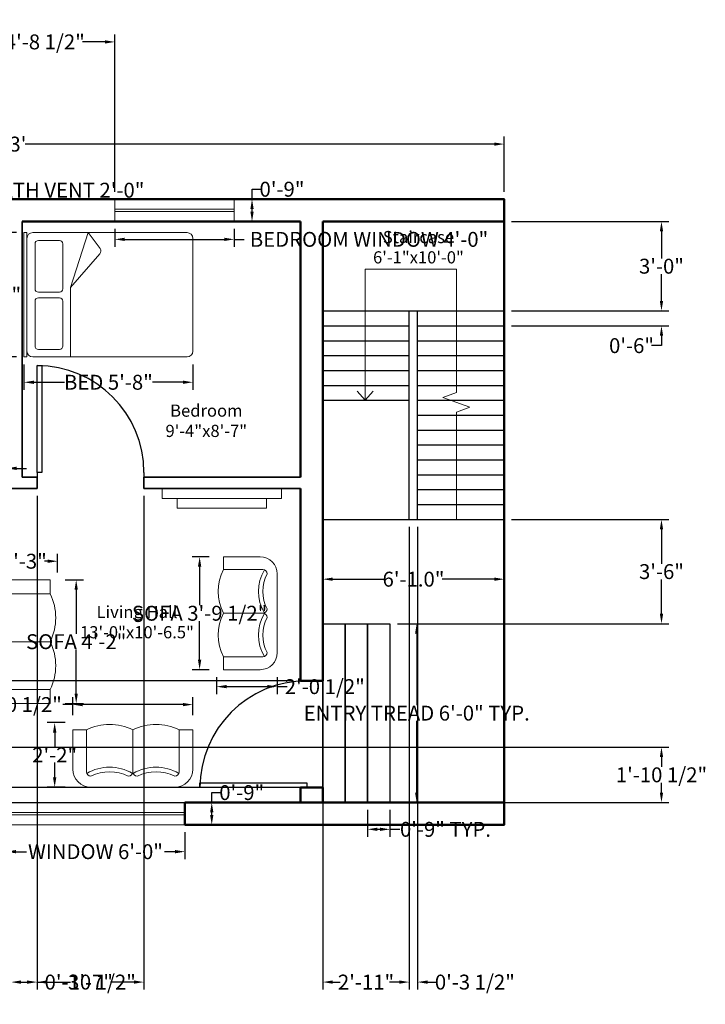
# Model space of a CAD drawing. Units: inches. Extents: x -59 to 502, y -260 to 136.
# Tile 8 of 8: x 226 to 502, y -260 to 136. Entities that reach past the tile are written whole.
import ezdxf

# ---------------------------------------------------------------- set-up
doc = ezdxf.new("R2010")
doc.units = ezdxf.units.IN
doc.header["$MEASUREMENT"] = 0
for name, color, linetype, lineweight in [('A-ANNO-DIMS', 2, 'Continuous', 18), ('A-ANNO-SYMB', 7, 'Continuous', 18), ('A-AREA-IDEN', 7, 'Continuous', 25), ('A-FLOR-CASE', 9, 'Continuous', 18), ('Beds', 122, 'Continuous', 18), ('Doors', 18, 'Continuous', 25), ('Inner wall', 11, 'Continuous', 35), ('Outer Wall', 10, 'Continuous', 50), ('Sofas', 84, 'Continuous', 18), ('Staircase', 200, 'Continuous', 25), ('Windows', 150, 'Continuous', 18)]:
    doc.layers.add(name, color=color, linetype=linetype, lineweight=lineweight)
doc.styles.get("Standard").update_dxf_attribs({"font": 'arial.ttf'})
doc.dimstyles.get("Standard").update_dxf_attribs({"dimtxt": 6, "dimasz": 4, "dimexe": 3, "dimexo": 3, "dimgap": 0.09, "dimtad": 0, "dimtih": 1, "dimtoh": 1, "dimdec": 1, "dimzin": 0, "dimdsep": 46, "dimlunit": 3, "dimtxsty": 'Standard', "dimcen": 0.09, "dimadec": 0, "dimazin": 0, "dimtfac": 1, "dimtdec": 1, "dimtofl": 0, "dimtmove": 0, "dimatfit": 3, "dimfxl": 1, "dimtolj": 1, "dimtzin": 0, "dimarcsym": 0})

# ---------------------------------------------------------------- blocks, each defined once
blk = doc.blocks.new('Window')
for p, q in [((868.39, 234.72), (940.39, 234.72)), ((868.39, 225.72), (868.39, 234.72)), ((940.39, 234.72), (940.39, 225.72)), ((868.39, 230.72), (940.39, 230.72)), ((940.39, 229.72), (868.39, 229.72)), ((940.39, 225.72), (868.39, 225.72))]:
    blk.add_line(p, q)
blk = doc.blocks.new('Window 2')
for p, q in [((928.89, 205.98), (976.89, 205.98)), ((928.89, 196.98), (928.89, 205.98)), ((976.89, 205.98), (976.89, 196.98)), ((928.89, 201.98), (976.89, 201.98)), ((976.89, 200.98), (928.89, 200.98)), ((976.89, 196.98), (928.89, 196.98))]:
    blk.add_line(p, q)
blk = doc.blocks.new('*D7')
at = {"layer": 'A-ANNO-DIMS', "color": 0, "lineweight": -2, "transparency": 16777216}
for p, q in [((25.46, 66.92), (25.46, 89.09)), ((421.46, 66.92), (421.46, 89.09)), ((29.46, 86.09), (218.28, 86.09)), ((417.46, 86.09), (228.64, 86.09))]:
    blk.add_line(p, q, dxfattribs=at)
at = {"layer": 'A-ANNO-DIMS', "color": 0, "transparency": 16777216}
for points in [[(29.46, 86.75), (29.46, 85.42), (25.46, 86.09)], [(417.46, 86.75), (417.46, 85.42), (421.46, 86.09)]]:
    blk.add_solid(points, dxfattribs=at)
at = {"layer": 'Defpoints', "color": 0, "transparency": 16777216}
for p in [(421.46, 86.09), (25.46, 63.92), (421.46, 63.92)]:
    blk.add_point(p, dxfattribs=at)
at = {"layer": 'A-ANNO-DIMS', "color": 0, "transparency": 16777216, "insert": (223.46, 86.09), "char_height": 6, "attachment_point": 5}
blk.add_mtext("\\A1;33'", dxfattribs=at)
blk = doc.blocks.new('*D8')
at = {"layer": 'A-ANNO-DIMS', "color": 0, "lineweight": -2, "transparency": 16777216}
for p, q in [((348.46, -68.08), (348.46, -92.13)), ((421.46, -68.08), (421.46, -92.13)), ((352.46, -89.13), (373.38, -89.13)), ((417.46, -89.13), (396.54, -89.13))]:
    blk.add_line(p, q, dxfattribs=at)
at = {"layer": 'A-ANNO-DIMS', "color": 0, "transparency": 16777216}
for points in [[(352.46, -88.47), (352.46, -89.8), (348.46, -89.13)], [(417.46, -88.47), (417.46, -89.8), (421.46, -89.13)]]:
    blk.add_solid(points, dxfattribs=at)
at = {"layer": 'Defpoints', "color": 0, "transparency": 16777216}
for p in [(348.46, -65.08), (421.46, -65.08), (421.46, -89.13)]:
    blk.add_point(p, dxfattribs=at)
at = {"layer": 'A-ANNO-DIMS', "color": 0, "transparency": 16777216, "insert": (384.96, -89.13), "char_height": 6, "attachment_point": 5}
blk.add_mtext('\\A1;6\'-1.0"', dxfattribs=at)
blk = doc.blocks.new('*U10')
for p, q in [((-40, 0), (-40, 6)), ((0, 0), (0, 6))]:
    blk.add_line(p, q)
blk.add_lwpolyline([(0, 0), (0, -40), (-1.75, -40), (-1.75, 0)], close=True)
blk.add_arc((0, 0), 40, 180, 270)
blk = doc.blocks.new('*U15')
for p, q in [((0, 0), (0, -6)), ((40, 0), (40, -6))]:
    blk.add_line(p, q)
blk.add_lwpolyline([(0, 0), (0, 40), (1.75, 40), (1.75, 0)], close=True)
blk.add_arc((0, 0), 40, 0, 90)
blk = doc.blocks.new('A$C164346CA')
for p, q in [((0, 2.035), (0, 2)), ((1.5, 2.035), (0, 2.035)), ((1.5, 2), (1.5, 2.035)), ((1.5, 2), (0, 2)), ((0, 1.93), (0, 0.07)), ((0.673, 1.902), (0.132, 1.902)), ((1.364, 1.902), (0.823, 1.902)), ((1.5, 0.07), (1.5, 1.93)), ((0.092, 1.862), (0.092, 1.607)), ((0.713, 1.607), (0.713, 1.862)), ((0.783, 1.862), (0.783, 1.607)), ((1.404, 1.607), (1.404, 1.862)), ((0.132, 1.567), (0.673, 1.567)), ((0.823, 1.567), (1.364, 1.567)), ((0.839, 1.476), (0, 1.476)), ((0.839, 1.476), (1.245, 1.12)), ((1.5, 1.261), (0.839, 1.476)), ((1.308, 1.117), (1.5, 1.261)), ((0.07, 0), (1.43, 0))]:
    blk.add_line(p, q)
for centre, radius, start, end in [((0.07, 1.93), 0.07, 90, 180), ((0.132, 1.862), 0.04, 90, 180), ((0.673, 1.862), 0.04, 0, 90), ((0.823, 1.862), 0.04, 90, 180), ((1.364, 1.862), 0.04, 0, 90), ((1.43, 1.93), 0.07, 0, 90), ((0.132, 1.607), 0.04, 180, 270), ((0.673, 1.607), 0.04, 270, 0), ((0.823, 1.607), 0.04, 180, 270), ((1.364, 1.607), 0.04, 270, 0), ((1.278, 1.158), 0.05, 228.6958, 306.7579), ((0.07, 0.07), 0.07, 180, 270), ((1.43, 0.07), 0.07, 270, 0)]:
    blk.add_arc(centre, radius, start, end)
blk = doc.blocks.new('A$C16D51D41')
for p, q in [((1.12, 0.69, -343.199), (0.2, 0.69, -343.199)), ((0, 0.49, -343.199), (0, 0.06, -343.199)), ((0.15, 0.52, -343.199), (0.15, 0.06, -343.199)), ((0.15, 0.06, -343.199), (0.15, 0.52, -343.199)), ((0.15, 0.52, -343.199), (0.15, 0.06, -343.199)), ((0.66, 0.06, -343.199), (0.66, 0.52, -343.199)), ((0.66, 0.52, -343.199), (0.66, 0.06, -343.199)), ((1.17, 0.52, -343.199), (1.17, 0.06, -343.199)), ((1.32, 0.06, -343.199), (1.32, 0.49, -343.199)), ((0, 0.06, -343.199), (0.15, 0.06, -343.199)), ((1.32, 0.06, -343.199), (1.17, 0.06, -343.199))]:
    blk.add_line(p, q)
for centre, radius, start, end in [((0.2, 0.49, -343.199), 0.2, 90, 180), ((1.12, 0.49, -343.199), 0.2, 0, 90), ((0.2, 0.52, -343.199), 0.05, 90, 180), ((0.405, 0.965, -343.199), 0.495, 239.4911, 300.5089), ((0.405, 0.965, -343.199), 0.445, 242.5861, 297.4139), ((0.61, 0.52, -343.199), 0.05, 0, 90), ((0.71, 0.52, -343.199), 0.05, 90, 180), ((0.915, 0.965, -343.199), 0.495, 239.4911, 300.5089), ((0.915, 0.965, -343.199), 0.445, 242.5861, 297.4139), ((1.12, 0.52, -343.199), 0.05, 0, 90), ((0.405, 0.572, -343.199), 0.572, 243.519, 296.481), ((0.915, 0.572, -343.199), 0.572, 243.519, 296.481)]:
    blk.add_arc(centre, radius, start, end)
blk = doc.blocks.new('ENTRY-STEP-72x9')
for p, q in [((0, 0), (0, 72)), ((0, 72), (9, 72)), ((9, 72), (9, 0)), ((9, 0), (0, 0))]:
    blk.add_line(p, q)
blk = doc.blocks.new('*D25')
at = {"layer": 'A-ANNO-DIMS', "color": 0, "lineweight": -2, "transparency": 16777216}
for p, q in [((247.8, -143.9), (247.8, -136.64)), ((296.18, -143.9), (296.18, -136.64)), ((247.8, -139.64), (243.8, -139.64)), ((292.18, -139.64), (251.8, -139.64))]:
    blk.add_line(p, q, dxfattribs=at)
at = {"layer": 'A-ANNO-DIMS', "color": 0, "transparency": 16777216}
for points in [[(251.8, -138.97), (251.8, -140.31), (247.8, -139.64)], [(292.18, -138.97), (292.18, -140.31), (296.18, -139.64)]]:
    blk.add_solid(points, dxfattribs=at)
at = {"layer": 'Defpoints', "color": 0, "transparency": 16777216}
for p in [(247.8, -139.64), (247.8, -146.9), (296.18, -146.9)]:
    blk.add_point(p, dxfattribs=at)
at = {"layer": 'A-ANNO-DIMS', "color": 0, "transparency": 16777216, "insert": (216.18, -139.64), "char_height": 6, "attachment_point": 5}
blk.add_mtext('\\A1;SOFA 4\'-0 1/2"', dxfattribs=at)
blk = doc.blocks.new('*D26')
at = {"layer": 'A-ANNO-DIMS', "color": 0, "lineweight": -2, "transparency": 16777216}
for p, q in [((244.8, -146.9), (237.54, -146.9)), ((240.54, -150.9), (240.54, -156.81)), ((240.54, -168.92), (240.54, -163.01)), ((244.8, -172.92), (237.54, -172.92))]:
    blk.add_line(p, q, dxfattribs=at)
at = {"layer": 'A-ANNO-DIMS', "color": 0, "transparency": 16777216}
for points in [[(239.87, -150.9), (241.21, -150.9), (240.54, -146.9)], [(239.87, -168.92), (241.21, -168.92), (240.54, -172.92)]]:
    blk.add_solid(points, dxfattribs=at)
at = {"layer": 'Defpoints', "color": 0, "transparency": 16777216}
for p in [(247.8, -146.9), (240.54, -172.92), (247.8, -172.92)]:
    blk.add_point(p, dxfattribs=at)
at = {"layer": 'A-ANNO-DIMS', "color": 0, "transparency": 16777216, "insert": (240.54, -159.91), "char_height": 6, "attachment_point": 5}
blk.add_mtext('\\A1;2\'-2"', dxfattribs=at)
blk = doc.blocks.new('*D27')
at = {"layer": 'A-ANNO-DIMS', "color": 0, "lineweight": -2, "transparency": 16777216}
for p, q in [((244.73, -89.38), (252.2, -89.38)), ((249.2, -93.38), (249.2, -111.12)), ((249.2, -135.24), (249.2, -117.51)), ((244.73, -139.24), (252.2, -139.24))]:
    blk.add_line(p, q, dxfattribs=at)
at = {"layer": 'A-ANNO-DIMS', "color": 0, "transparency": 16777216}
for points in [[(248.54, -93.38), (249.87, -93.38), (249.2, -89.38)], [(248.54, -135.24), (249.87, -135.24), (249.2, -139.24)]]:
    blk.add_solid(points, dxfattribs=at)
at = {"layer": 'Defpoints', "color": 0, "transparency": 16777216}
for p in [(241.73, -89.38), (249.2, -89.38), (241.73, -139.24)]:
    blk.add_point(p, dxfattribs=at)
at = {"layer": 'A-ANNO-DIMS', "color": 0, "transparency": 16777216, "insert": (249.2, -114.31), "char_height": 6, "attachment_point": 5}
blk.add_mtext('\\A1;SOFA 4\'-2"', dxfattribs=at)
blk = doc.blocks.new('*D28')
at = {"layer": 'A-ANNO-DIMS', "color": 0, "lineweight": -2, "transparency": 16777216}
for p, q in [((214.91, -86.38), (214.91, -78.9)), ((241.73, -86.38), (241.73, -78.9)), ((218.91, -81.9), (220.2, -81.9)), ((237.73, -81.9), (236.43, -81.9))]:
    blk.add_line(p, q, dxfattribs=at)
at = {"layer": 'A-ANNO-DIMS', "color": 0, "transparency": 16777216}
for points in [[(218.91, -81.24), (218.91, -82.57), (214.91, -81.9)], [(237.73, -81.24), (237.73, -82.57), (241.73, -81.9)]]:
    blk.add_solid(points, dxfattribs=at)
at = {"layer": 'Defpoints', "color": 0, "transparency": 16777216}
for p in [(214.91, -81.9), (214.91, -89.38), (241.73, -89.38)]:
    blk.add_point(p, dxfattribs=at)
at = {"layer": 'A-ANNO-DIMS', "color": 0, "transparency": 16777216, "insert": (228.32, -81.9), "char_height": 6, "attachment_point": 5}
blk.add_mtext('\\A1;2\'-3"', dxfattribs=at)
blk = doc.blocks.new('*D29')
at = {"layer": 'A-ANNO-DIMS', "color": 0, "lineweight": -2, "transparency": 16777216}
for p, q in [((302.7, -80.12), (295.88, -80.12)), ((298.88, -84.12), (298.88, -99.66)), ((298.88, -121.59), (298.88, -106.05)), ((302.7, -125.59), (295.88, -125.59))]:
    blk.add_line(p, q, dxfattribs=at)
at = {"layer": 'A-ANNO-DIMS', "color": 0, "transparency": 16777216}
for points in [[(298.21, -84.12), (299.54, -84.12), (298.88, -80.12)], [(298.21, -121.59), (299.54, -121.59), (298.88, -125.59)]]:
    blk.add_solid(points, dxfattribs=at)
at = {"layer": 'Defpoints', "color": 0, "transparency": 16777216}
for p in [(305.7, -80.12), (298.88, -125.59), (305.7, -125.59)]:
    blk.add_point(p, dxfattribs=at)
at = {"layer": 'A-ANNO-DIMS', "color": 0, "transparency": 16777216, "insert": (298.88, -102.86), "char_height": 6, "attachment_point": 5}
blk.add_mtext('\\A1;SOFA 3\'-9 1/2"', dxfattribs=at)
blk = doc.blocks.new('*D30')
at = {"layer": 'A-ANNO-DIMS', "color": 0, "lineweight": -2, "transparency": 16777216}
for p, q in [((305.7, -128.59), (305.7, -135.41)), ((330.15, -128.59), (330.15, -135.41)), ((309.7, -132.41), (326.15, -132.41)), ((330.15, -132.41), (334.15, -132.41))]:
    blk.add_line(p, q, dxfattribs=at)
at = {"layer": 'A-ANNO-DIMS', "color": 0, "transparency": 16777216}
for points in [[(309.7, -131.74), (309.7, -133.07), (305.7, -132.41)], [(326.15, -131.74), (326.15, -133.07), (330.15, -132.41)]]:
    blk.add_solid(points, dxfattribs=at)
at = {"layer": 'Defpoints', "color": 0, "transparency": 16777216}
for p in [(305.7, -125.59), (330.15, -125.59), (330.15, -132.41)]:
    blk.add_point(p, dxfattribs=at)
at = {"layer": 'A-ANNO-DIMS', "color": 0, "transparency": 16777216, "insert": (349.26, -132.41), "char_height": 6, "attachment_point": 5}
blk.add_mtext('\\A1;2\'-0 1/2"', dxfattribs=at)
blk = doc.blocks.new('*D31')
at = {"layer": 'A-ANNO-DIMS', "color": 0, "lineweight": -2, "transparency": 16777216}
for p, q in [((378.46, -107.08), (389.26, -107.08)), ((386.26, -111.08), (386.26, -139.92)), ((386.26, -175.08), (386.26, -146.23)), ((378.46, -179.08), (389.26, -179.08))]:
    blk.add_line(p, q, dxfattribs=at)
at = {"layer": 'A-ANNO-DIMS', "color": 0, "transparency": 16777216}
for points in [[(385.59, -111.08), (386.93, -111.08), (386.26, -107.08)], [(385.59, -175.08), (386.93, -175.08), (386.26, -179.08)]]:
    blk.add_solid(points, dxfattribs=at)
at = {"layer": 'Defpoints', "color": 0, "transparency": 16777216}
for p in [(375.46, -107.08), (386.26, -107.08), (375.46, -179.08)]:
    blk.add_point(p, dxfattribs=at)
at = {"layer": 'A-ANNO-DIMS', "color": 0, "transparency": 16777216, "insert": (386.26, -143.08), "char_height": 6, "attachment_point": 5}
blk.add_mtext('\\A1;ENTRY TREAD 6\'-0" TYP.', dxfattribs=at)
blk = doc.blocks.new('*D32')
at = {"layer": 'A-ANNO-DIMS', "color": 0, "lineweight": -2, "transparency": 16777216}
for p, q in [((366.46, -182.08), (366.46, -192.88)), ((375.46, -182.08), (375.46, -192.88)), ((370.46, -189.88), (371.46, -189.88)), ((375.46, -189.88), (379.46, -189.88))]:
    blk.add_line(p, q, dxfattribs=at)
at = {"layer": 'A-ANNO-DIMS', "color": 0, "transparency": 16777216}
for points in [[(370.46, -189.21), (370.46, -190.54), (366.46, -189.88)], [(371.46, -189.21), (371.46, -190.54), (375.46, -189.88)]]:
    blk.add_solid(points, dxfattribs=at)
at = {"layer": 'Defpoints', "color": 0, "transparency": 16777216}
for p in [(366.46, -179.08), (375.46, -179.08), (375.46, -189.88)]:
    blk.add_point(p, dxfattribs=at)
at = {"layer": 'A-ANNO-DIMS', "color": 0, "transparency": 16777216, "insert": (397.84, -189.88), "char_height": 6, "attachment_point": 5}
blk.add_mtext('\\A1;0\'-9" TYP.', dxfattribs=at)
blk = doc.blocks.new('*D35')
at = {"layer": 'A-ANNO-DIMS', "color": 0, "lineweight": -2, "transparency": 16777216}
for p, q in [((184.38, 66.92), (184.38, 70.52)), ((188.38, 67.52), (204.38, 67.52)), ((208.38, 66.92), (208.38, 70.52)), ((208.38, 67.52), (212.38, 67.52))]:
    blk.add_line(p, q, dxfattribs=at)
at = {"layer": 'A-ANNO-DIMS', "color": 0, "transparency": 16777216}
for points in [[(188.38, 68.19), (188.38, 66.86), (184.38, 67.52)], [(204.38, 68.19), (204.38, 66.86), (208.38, 67.52)]]:
    blk.add_solid(points, dxfattribs=at)
at = {"layer": 'Defpoints', "color": 0, "transparency": 16777216}
for p in [(208.38, 67.52), (184.38, 63.92), (208.38, 63.92)]:
    blk.add_point(p, dxfattribs=at)
at = {"layer": 'A-ANNO-DIMS', "color": 0, "transparency": 16777216, "insert": (244.99, 67.52), "char_height": 6, "attachment_point": 5}
blk.add_mtext('\\A1;BATH VENT 2\'-0"', dxfattribs=at)
blk = doc.blocks.new('*D37')
at = {"layer": 'A-ANNO-DIMS', "color": 0, "lineweight": -2, "transparency": 16777216}
for p, q in [((220.96, -191.08), (220.96, -201.88)), ((292.96, -191.08), (292.96, -201.88)), ((224.96, -198.88), (229.22, -198.88)), ((288.96, -198.88), (284.7, -198.88))]:
    blk.add_line(p, q, dxfattribs=at)
at = {"layer": 'A-ANNO-DIMS', "color": 0, "transparency": 16777216}
for points in [[(224.96, -198.21), (224.96, -199.54), (220.96, -198.88)], [(288.96, -198.21), (288.96, -199.54), (292.96, -198.88)]]:
    blk.add_solid(points, dxfattribs=at)
at = {"layer": 'Defpoints', "color": 0, "transparency": 16777216}
for p in [(220.96, -188.08), (292.96, -188.08), (292.96, -198.88)]:
    blk.add_point(p, dxfattribs=at)
at = {"layer": 'A-ANNO-DIMS', "color": 0, "transparency": 16777216, "insert": (256.96, -198.88), "char_height": 6, "attachment_point": 5}
blk.add_mtext('\\A1;WINDOW 6\'-0"', dxfattribs=at)
blk = doc.blocks.new('*D38')
at = {"layer": 'A-ANNO-DIMS', "color": 0, "lineweight": -2, "transparency": 16777216}
for p, q in [((303.76, -179.08), (303.76, -175.08)), ((303.76, -175.08), (307.76, -175.08)), ((295.96, -179.08), (306.76, -179.08)), ((303.76, -184.08), (303.76, -183.08)), ((295.96, -188.08), (306.76, -188.08))]:
    blk.add_line(p, q, dxfattribs=at)
at = {"layer": 'A-ANNO-DIMS', "color": 0, "transparency": 16777216}
for points in [[(303.09, -183.08), (304.43, -183.08), (303.76, -179.08)], [(303.09, -184.08), (304.43, -184.08), (303.76, -188.08)]]:
    blk.add_solid(points, dxfattribs=at)
at = {"layer": 'Defpoints', "color": 0, "transparency": 16777216}
for p in [(292.96, -179.08), (303.76, -179.08), (292.96, -188.08)]:
    blk.add_point(p, dxfattribs=at)
at = {"layer": 'A-ANNO-DIMS', "color": 0, "transparency": 16777216, "insert": (315.83, -175.08), "char_height": 6, "attachment_point": 5}
blk.add_mtext('\\A1;0\'-9"', dxfattribs=at)
blk = doc.blocks.new('*D39')
at = {"layer": 'A-ANNO-DIMS', "color": 0, "lineweight": -2, "transparency": 16777216}
for p, q in [((264.77, 51.92), (264.77, 44.72)), ((312.77, 51.92), (312.77, 44.72)), ((268.77, 47.72), (308.77, 47.72)), ((312.77, 47.72), (316.77, 47.72))]:
    blk.add_line(p, q, dxfattribs=at)
at = {"layer": 'A-ANNO-DIMS', "color": 0, "transparency": 16777216}
for points in [[(268.77, 48.39), (268.77, 47.06), (264.77, 47.72)], [(308.77, 48.39), (308.77, 47.06), (312.77, 47.72)]]:
    blk.add_solid(points, dxfattribs=at)
at = {"layer": 'Defpoints', "color": 0, "transparency": 16777216}
for p in [(264.77, 54.92), (312.77, 54.92), (312.77, 47.72)]:
    blk.add_point(p, dxfattribs=at)
at = {"layer": 'A-ANNO-DIMS', "color": 0, "transparency": 16777216, "insert": (367.07, 47.72), "char_height": 6, "attachment_point": 5}
blk.add_mtext('\\A1;BEDROOM WINDOW 4\'-0"', dxfattribs=at)
blk = doc.blocks.new('*D40')
at = {"layer": 'A-ANNO-DIMS', "color": 0, "lineweight": -2, "transparency": 16777216}
for p, q in [((319.97, 63.92), (319.97, 67.92)), ((319.97, 67.92), (323.97, 67.92)), ((315.77, 63.92), (322.97, 63.92)), ((319.97, 58.92), (319.97, 59.92)), ((315.77, 54.92), (322.97, 54.92))]:
    blk.add_line(p, q, dxfattribs=at)
at = {"layer": 'A-ANNO-DIMS', "color": 0, "transparency": 16777216}
for points in [[(319.3, 59.92), (320.64, 59.92), (319.97, 63.92)], [(319.3, 58.92), (320.64, 58.92), (319.97, 54.92)]]:
    blk.add_solid(points, dxfattribs=at)
at = {"layer": 'Defpoints', "color": 0, "transparency": 16777216}
for p in [(312.77, 63.92), (319.97, 63.92), (312.77, 54.92)]:
    blk.add_point(p, dxfattribs=at)
at = {"layer": 'A-ANNO-DIMS', "color": 0, "transparency": 16777216, "insert": (332.03, 67.92), "char_height": 6, "attachment_point": 5}
blk.add_mtext('\\A1;0\'-9"', dxfattribs=at)
blk = doc.blocks.new('*D47')
at = {"layer": 'A-ANNO-DIMS', "color": 0, "lineweight": -2, "transparency": 16777216}
for p, q in [((228.19, -2.64), (228.19, -12.83)), ((296.14, -2.64), (296.14, -12.83)), ((232.19, -9.83), (244.45, -9.83)), ((292.14, -9.83), (279.88, -9.83))]:
    blk.add_line(p, q, dxfattribs=at)
at = {"layer": 'A-ANNO-DIMS', "color": 0, "transparency": 16777216}
for points in [[(232.19, -9.16), (232.19, -10.5), (228.19, -9.83)], [(292.14, -9.16), (292.14, -10.5), (296.14, -9.83)]]:
    blk.add_solid(points, dxfattribs=at)
at = {"layer": 'Defpoints', "color": 0, "transparency": 16777216}
for p in [(228.19, 0.36), (296.14, 0.36), (228.19, -9.83)]:
    blk.add_point(p, dxfattribs=at)
at = {"layer": 'A-ANNO-DIMS', "color": 0, "transparency": 16777216, "insert": (262.17, -9.83), "char_height": 6, "attachment_point": 5}
blk.add_mtext('\\A1;BED 5\'-8"', dxfattribs=at)
blk = doc.blocks.new('*D48')
at = {"layer": 'A-ANNO-DIMS', "color": 0, "lineweight": -2, "transparency": 16777216}
for p, q in [((225.19, 50.45), (215, 50.45)), ((218, 46.45), (218, 28.51)), ((218, 4.36), (218, 22.31)), ((225.19, 0.36), (215, 0.36))]:
    blk.add_line(p, q, dxfattribs=at)
at = {"layer": 'A-ANNO-DIMS', "color": 0, "transparency": 16777216}
for points in [[(217.33, 46.45), (218.66, 46.45), (218, 50.45)], [(217.33, 4.36), (218.66, 4.36), (218, 0.36)]]:
    blk.add_solid(points, dxfattribs=at)
at = {"layer": 'Defpoints', "color": 0, "transparency": 16777216}
for p in [(218, 50.45), (228.19, 50.45), (228.19, 0.36)]:
    blk.add_point(p, dxfattribs=at)
at = {"layer": 'A-ANNO-DIMS', "color": 0, "transparency": 16777216, "insert": (218, 25.41), "char_height": 6, "attachment_point": 5}
blk.add_mtext('\\A1;4\'-2"', dxfattribs=at)
blk = doc.blocks.new('*D56')
at = {"layer": 'A-ANNO-DIMS', "color": 0, "lineweight": -2, "transparency": 16777216}
for p, q in [((201.1, -42.98), (201.1, -47.5)), ((221.19, -42.98), (221.19, -47.5)), ((197.1, -44.5), (193.1, -44.5)), ((225.19, -44.5), (229.19, -44.5))]:
    blk.add_line(p, q, dxfattribs=at)
at = {"layer": 'A-ANNO-DIMS', "color": 0, "transparency": 16777216}
for points in [[(197.1, -43.83), (197.1, -45.16), (201.1, -44.5)], [(225.19, -43.83), (225.19, -45.16), (221.19, -44.5)]]:
    blk.add_solid(points, dxfattribs=at)
at = {"layer": 'Defpoints', "color": 0, "transparency": 16777216}
for p in [(201.1, -39.98), (221.19, -39.98), (221.19, -44.5)]:
    blk.add_point(p, dxfattribs=at)
at = {"layer": 'A-ANNO-DIMS', "color": 0, "transparency": 16777216, "insert": (211.15, -44.5), "char_height": 6, "attachment_point": 5}
blk.add_mtext('\\A1;1\'-8"', dxfattribs=at)
blk = doc.blocks.new('*D58')
at = {"layer": 'A-ANNO-DIMS', "color": 0, "lineweight": -2, "transparency": 16777216}
for p, q in [((208.38, 66.92), (208.38, 130.25)), ((212.38, 127.25), (221.4, 127.25)), ((260.77, 127.25), (251.75, 127.25)), ((264.77, 66.92), (264.77, 130.25))]:
    blk.add_line(p, q, dxfattribs=at)
at = {"layer": 'A-ANNO-DIMS', "color": 0, "transparency": 16777216}
for points in [[(212.38, 127.91), (212.38, 126.58), (208.38, 127.25)], [(260.77, 127.91), (260.77, 126.58), (264.77, 127.25)]]:
    blk.add_solid(points, dxfattribs=at)
at = {"layer": 'Defpoints', "color": 0, "transparency": 16777216}
for p in [(264.77, 127.25), (208.38, 63.92), (264.77, 63.92)]:
    blk.add_point(p, dxfattribs=at)
at = {"layer": 'A-ANNO-DIMS', "color": 0, "transparency": 16777216, "insert": (236.57, 127.25), "char_height": 6, "attachment_point": 5}
blk.add_mtext('\\A1;4\'-8 1/2"', dxfattribs=at)
blk = doc.blocks.new('*D62')
at = {"layer": 'A-ANNO-DIMS', "color": 0, "lineweight": -2, "transparency": 16777216}
for p, q in [((424.46, 54.92), (487.78, 54.92)), ((484.78, 50.92), (484.78, 40.08)), ((484.78, 22.92), (484.78, 33.77)), ((424.46, 18.92), (487.78, 18.92))]:
    blk.add_line(p, q, dxfattribs=at)
at = {"layer": 'A-ANNO-DIMS', "color": 0, "transparency": 16777216}
for points in [[(484.12, 50.92), (485.45, 50.92), (484.78, 54.92)], [(484.12, 22.92), (485.45, 22.92), (484.78, 18.92)]]:
    blk.add_solid(points, dxfattribs=at)
at = {"layer": 'Defpoints', "color": 0, "transparency": 16777216}
for p in [(421.46, 54.92), (421.46, 18.92), (484.78, 18.92)]:
    blk.add_point(p, dxfattribs=at)
at = {"layer": 'A-ANNO-DIMS', "color": 0, "transparency": 16777216, "insert": (484.78, 36.92), "char_height": 6, "attachment_point": 5}
blk.add_mtext('\\A1;3\'-0"', dxfattribs=at)
blk = doc.blocks.new('*D63')
at = {"layer": 'A-ANNO-DIMS', "color": 0, "lineweight": -2, "transparency": 16777216}
for p, q in [((484.78, 22.92), (484.78, 26.92)), ((424.46, 18.92), (487.78, 18.92)), ((424.46, 12.92), (487.78, 12.92)), ((484.78, 8.92), (484.78, 4.92)), ((484.78, 4.92), (480.78, 4.92))]:
    blk.add_line(p, q, dxfattribs=at)
at = {"layer": 'A-ANNO-DIMS', "color": 0, "transparency": 16777216}
for points in [[(484.12, 22.92), (485.45, 22.92), (484.78, 18.92)], [(484.12, 8.92), (485.45, 8.92), (484.78, 12.92)]]:
    blk.add_solid(points, dxfattribs=at)
at = {"layer": 'Defpoints', "color": 0, "transparency": 16777216}
for p in [(421.46, 18.92), (421.46, 12.92), (484.78, 12.92)]:
    blk.add_point(p, dxfattribs=at)
at = {"layer": 'A-ANNO-DIMS', "color": 0, "transparency": 16777216, "insert": (472.72, 4.92), "char_height": 6, "attachment_point": 5}
blk.add_mtext('\\A1;0\'-6"', dxfattribs=at)
blk = doc.blocks.new('*D64')
at = {"layer": 'A-ANNO-DIMS', "color": 0, "lineweight": -2, "transparency": 16777216}
for p, q in [((348.46, -68.08), (348.46, -254.4)), ((383.26, -68.08), (383.26, -254.4)), ((352.46, -251.4), (355.41, -251.4)), ((379.26, -251.4), (376.31, -251.4))]:
    blk.add_line(p, q, dxfattribs=at)
at = {"layer": 'A-ANNO-DIMS', "color": 0, "transparency": 16777216}
for points in [[(352.46, -250.74), (352.46, -252.07), (348.46, -251.4)], [(379.26, -250.74), (379.26, -252.07), (383.26, -251.4)]]:
    blk.add_solid(points, dxfattribs=at)
at = {"layer": 'Defpoints', "color": 0, "transparency": 16777216}
for p in [(348.46, -65.08), (383.26, -65.08), (383.26, -251.4)]:
    blk.add_point(p, dxfattribs=at)
at = {"layer": 'A-ANNO-DIMS', "color": 0, "transparency": 16777216, "insert": (365.86, -251.4), "char_height": 6, "attachment_point": 5}
blk.add_mtext('\\A1;2\'-11"', dxfattribs=at)
blk = doc.blocks.new('*D65')
at = {"layer": 'A-ANNO-DIMS', "color": 0, "lineweight": -2, "transparency": 16777216}
for p, q in [((383.26, -68.08), (383.26, -254.4)), ((386.62, -68.08), (386.62, -254.4)), ((379.26, -251.4), (375.26, -251.4)), ((390.62, -251.4), (394.62, -251.4))]:
    blk.add_line(p, q, dxfattribs=at)
at = {"layer": 'A-ANNO-DIMS', "color": 0, "transparency": 16777216}
for points in [[(379.26, -250.74), (379.26, -252.07), (383.26, -251.4)], [(390.62, -250.74), (390.62, -252.07), (386.62, -251.4)]]:
    blk.add_solid(points, dxfattribs=at)
at = {"layer": 'Defpoints', "color": 0, "transparency": 16777216}
for p in [(383.26, -65.08), (386.62, -65.08), (386.62, -251.4)]:
    blk.add_point(p, dxfattribs=at)
at = {"layer": 'A-ANNO-DIMS', "color": 0, "transparency": 16777216, "insert": (409.67, -251.4), "char_height": 6, "attachment_point": 5}
blk.add_mtext('\\A1;0\'-3 1/2"', dxfattribs=at)
blk = doc.blocks.new('*D66')
at = {"layer": 'A-ANNO-DIMS', "color": 0, "lineweight": -2, "transparency": 16777216}
for p, q in [((336.46, -130.08), (-40.87, -130.08)), ((-37.87, -134.08), (-37.87, -148.42)), ((-37.87, -169.08), (-37.87, -154.73)), ((336.46, -173.08), (-40.87, -173.08))]:
    blk.add_line(p, q, dxfattribs=at)
at = {"layer": 'A-ANNO-DIMS', "color": 0, "transparency": 16777216}
for points in [[(-38.53, -134.08), (-37.2, -134.08), (-37.87, -130.08)], [(-38.53, -169.08), (-37.2, -169.08), (-37.87, -173.08)]]:
    blk.add_solid(points, dxfattribs=at)
at = {"layer": 'Defpoints', "color": 0, "transparency": 16777216}
for p in [(339.46, -130.08), (-37.87, -173.08), (339.46, -173.08)]:
    blk.add_point(p, dxfattribs=at)
at = {"layer": 'A-ANNO-DIMS', "color": 0, "transparency": 16777216, "insert": (-37.87, -151.58), "char_height": 6, "attachment_point": 5}
blk.add_mtext('\\A1;3\'-7"', dxfattribs=at)
blk = doc.blocks.new('*D67')
at = {"layer": 'A-ANNO-DIMS', "color": 0, "lineweight": -2, "transparency": 16777216}
for p, q in [((424.46, -65.08), (487.78, -65.08)), ((484.78, -69.08), (484.78, -82.92)), ((484.78, -103.08), (484.78, -89.23)), ((378.46, -107.08), (487.78, -107.08))]:
    blk.add_line(p, q, dxfattribs=at)
at = {"layer": 'A-ANNO-DIMS', "color": 0, "transparency": 16777216}
for points in [[(484.12, -69.08), (485.45, -69.08), (484.78, -65.08)], [(484.12, -103.08), (485.45, -103.08), (484.78, -107.08)]]:
    blk.add_solid(points, dxfattribs=at)
at = {"layer": 'Defpoints', "color": 0, "transparency": 16777216}
for p in [(421.46, -65.08), (375.46, -107.08), (484.78, -107.08)]:
    blk.add_point(p, dxfattribs=at)
at = {"layer": 'A-ANNO-DIMS', "color": 0, "transparency": 16777216, "insert": (484.78, -86.08), "char_height": 6, "attachment_point": 5}
blk.add_mtext('\\A1;3\'-6"', dxfattribs=at)
blk = doc.blocks.new('*D70')
at = {"layer": 'A-ANNO-DIMS', "color": 0, "lineweight": -2, "transparency": 16777216}
for p, q in [((233.46, -55.58), (233.46, -254.4)), ((276.46, -55.58), (276.46, -254.4)), ((237.46, -251.4), (246.9, -251.4)), ((272.46, -251.4), (263.02, -251.4))]:
    blk.add_line(p, q, dxfattribs=at)
at = {"layer": 'A-ANNO-DIMS', "color": 0, "transparency": 16777216}
for points in [[(237.46, -250.74), (237.46, -252.07), (233.46, -251.4)], [(272.46, -250.74), (272.46, -252.07), (276.46, -251.4)]]:
    blk.add_solid(points, dxfattribs=at)
at = {"layer": 'Defpoints', "color": 0, "transparency": 16777216}
for p in [(233.46, -52.58), (276.46, -52.58), (276.46, -251.4)]:
    blk.add_point(p, dxfattribs=at)
at = {"layer": 'A-ANNO-DIMS', "color": 0, "transparency": 16777216, "insert": (254.96, -251.4), "char_height": 6, "attachment_point": 5}
blk.add_mtext('\\A1;3\'-7"', dxfattribs=at)
blk = doc.blocks.new('*D73')
at = {"layer": 'A-ANNO-DIMS', "color": 0, "lineweight": -2, "transparency": 16777216}
for p, q in [((116.34, -156.78), (487.78, -156.78)), ((484.78, -160.78), (484.78, -164.74)), ((484.78, -175.08), (484.78, -171.12)), ((116.34, -179.08), (487.78, -179.08))]:
    blk.add_line(p, q, dxfattribs=at)
at = {"layer": 'A-ANNO-DIMS', "color": 0, "transparency": 16777216}
for points in [[(484.12, -160.78), (485.45, -160.78), (484.78, -156.78)], [(484.12, -175.08), (485.45, -175.08), (484.78, -179.08)]]:
    blk.add_solid(points, dxfattribs=at)
at = {"layer": 'Defpoints', "color": 0, "transparency": 16777216}
for p in [(113.34, -156.78), (113.34, -179.08), (484.78, -179.08)]:
    blk.add_point(p, dxfattribs=at)
at = {"layer": 'A-ANNO-DIMS', "color": 0, "transparency": 16777216, "insert": (484.78, -167.93), "char_height": 6, "attachment_point": 5}
blk.add_mtext('\\A1;1\'-10 1/2"', dxfattribs=at)
blk = doc.blocks.new('*D75')
at = {"layer": 'A-ANNO-DIMS', "color": 0, "lineweight": -2, "transparency": 16777216}
for p, q in [((222.96, -55.58), (222.96, -254.4)), ((233.46, -55.58), (233.46, -254.4)), ((226.96, -251.4), (229.46, -251.4)), ((233.46, -251.4), (237.46, -251.4))]:
    blk.add_line(p, q, dxfattribs=at)
at = {"layer": 'A-ANNO-DIMS', "color": 0, "transparency": 16777216}
for points in [[(226.96, -250.74), (226.96, -252.07), (222.96, -251.4)], [(229.46, -250.74), (229.46, -252.07), (233.46, -251.4)]]:
    blk.add_solid(points, dxfattribs=at)
at = {"layer": 'Defpoints', "color": 0, "transparency": 16777216}
for p in [(222.96, -52.58), (233.46, -52.58), (233.46, -251.4)]:
    blk.add_point(p, dxfattribs=at)
at = {"layer": 'A-ANNO-DIMS', "color": 0, "transparency": 16777216, "insert": (254.85, -251.4), "char_height": 6, "attachment_point": 5}
blk.add_mtext('\\A1;0\'-10 1/2"', dxfattribs=at)

msp = doc.modelspace()

# ---------------------------------------------------------------- linework, layer by layer
at = {"layer": 'A-ANNO-SYMB'}
for q in [(362.26, -13.36), (368.71, -13.36)]:
    msp.add_line((365.48, -17.08), q, dxfattribs=at)
msp.add_lwpolyline([(365.48, -17.08), (365.48, 35.68), (402.21, 35.68), (402.21, -13.98), (396.81, -15.94), (407.61, -19.87), (402.21, -21.84), (402.21, -65.08)], dxfattribs=at)
at = {"layer": 'A-FLOR-CASE'}
for p, q in [((283.8, -52.58), (283.8, -56.58)), ((331.8, -52.58), (331.8, -56.58)), ((283.8, -56.58), (331.8, -56.58)), ((289.8, -56.58), (289.8, -60.58)), ((325.8, -56.58), (325.8, -60.58)), ((289.8, -60.58), (325.8, -60.58))]:
    msp.add_line(p, q, dxfattribs=at)
at = {"layer": 'Inner wall'}
for p, q in [((227.46, -48.08), (227.46, 54.92)), ((227.46, -48.08), (233.46, -48.08)), ((233.46, -52.58), (233.46, -48.08)), ((276.46, -52.58), (276.46, -48.08)), ((276.46, -48.08), (339.46, -48.08)), ((222.96, -52.58), (233.46, -52.58)), ((276.46, -52.58), (339.46, -52.58))]:
    msp.add_line(p, q, dxfattribs=at)
at = {"layer": 'Outer Wall'}
for p, q in [((227.46, 54.92), (339.46, 54.92)), ((339.46, -48.08), (339.46, 54.92)), ((348.46, 54.92), (421.46, 54.92)), ((348.46, -130.08), (348.46, 54.92)), ((339.46, -130.08), (339.46, -52.58)), ((348.46, -130.08), (339.46, -130.08)), ((339.46, -179.08), (339.46, -173.08)), ((348.46, -173.08), (339.46, -173.08)), ((348.46, -179.08), (348.46, -173.08)), ((348.46, -179.08), (292.96, -179.08)), ((292.96, -188.08), (292.96, -179.08)), ((421.46, -179.08), (348.46, -179.08))]:
    msp.add_line(p, q, dxfattribs=at)
msp.add_lwpolyline([(220.96, -188.08), (25.46, -188.08), (25.46, 63.92), (421.46, 63.92), (421.46, -188.08), (292.96, -188.08)], dxfattribs=at)
at = {"layer": 'Staircase'}
for p, q in [((348.46, 18.92), (421.46, 18.92)), ((383.26, -65.08), (383.26, 18.92)), ((386.62, -65.08), (386.62, 18.92)), ((348.46, 12.92), (383.26, 12.92)), ((386.62, 12.92), (421.46, 12.92)), ((348.46, 6.92), (383.26, 6.92)), ((386.62, 6.92), (421.46, 6.92)), ((348.46, 0.92), (383.26, 0.92)), ((386.62, 0.92), (421.46, 0.92)), ((348.46, -5.08), (383.26, -5.08)), ((386.62, -5.08), (421.46, -5.08)), ((348.46, -11.08), (383.26, -11.08)), ((386.62, -11.08), (421.46, -11.08)), ((348.46, -17.08), (383.26, -17.08)), ((386.62, -17.08), (421.46, -17.08)), ((386.62, -23.08), (421.46, -23.08)), ((386.62, -29.08), (421.46, -29.08)), ((386.62, -35.08), (421.46, -35.08)), ((386.62, -41.08), (421.46, -41.08)), ((386.62, -47.08), (421.46, -47.08)), ((386.62, -53.08), (421.46, -53.08)), ((386.62, -59.08), (421.46, -59.08)), ((348.46, -65.08), (421.46, -65.08))]:
    msp.add_line(p, q, dxfattribs=at)
msp.add_lwpolyline([(357.46, -179.08), (348.46, -179.08), (348.46, -107.08), (357.46, -107.08)], close=True, dxfattribs=at)

# ---------------------------------------------------------------- block references
at = {"layer": 'Beds', "xscale": 33.39342335215582, "yscale": 33.39342335215582, "zscale": 33.39342335215582, "rotation": 90}
msp.add_blockref('A$C164346CA', (296.14, 0.36), dxfattribs=at)
at = {"layer": 'Doors', "xscale": 1.074999999999997, "yscale": 1.074999999999997, "zscale": 1.074999999999997}
msp.add_blockref('*U15', (233.46, -46.13), dxfattribs=at)
at = {"layer": 'Doors', "xscale": 1.074999999999999, "yscale": 1.074999999999999, "zscale": 1.074999999999999, "rotation": 270}
msp.add_blockref('*U10', (342.01, -173.08), dxfattribs=at)
at = {"layer": 'Sofas'}
for p, xscale, yscale, zscale, rotation in [((306.39, -80.12, 11820.07), 34.44086971581397, 34.44086971581397, 34.44086971581397, 270), ((240.97, -139.24, 12962.92), 37.77085078039113, 37.77085078039113, 37.77085078039113, 90), ((296.18, -147.63, 12579.82), 36.65459777142213, 36.65459777142213, 36.65459777142213, 180)]:
    msp.add_blockref('A$C16D51D41', p, dxfattribs=dict(at, xscale=xscale, yscale=yscale, zscale=zscale, rotation=rotation))
at = {"layer": 'Staircase'}
for p in [(357.46, -179.08), (366.46, -179.08)]:
    msp.add_blockref('ENTRY-STEP-72x9', p, dxfattribs=at)
at = {"layer": 'Windows'}
for name, p in [('Window 2', (-664.12, -142.05)), ('Window', (-647.43, -413.8))]:
    msp.add_blockref(name, p, dxfattribs=at)

# ---------------------------------------------------------------- texts
at = {"layer": 'A-AREA-IDEN', "char_height": 4.898, "attachment_point": 1}
for s, insert in [('\\pxqc;Staircase\\P6\'-1"x10\'-0"', (-583.16, 51.1)), ('\\pxqc;Bedroom \\P9\'-4"x8\'-7"', (-668.55, -18.8)), ('\\pxqc;Living Hall\\P13\'-0"x10\'-6.5"', (-696.45, -99.89))]:
    msp.add_mtext_dynamic_manual_height_columns(s, width=1940.2373, gutter_width=24.49, heights=[0], dxfattribs=dict(at, insert=insert))

# ---------------------------------------------------------------- dimensions: what is measured, and where the dimension line sits
at = {"layer": 'A-ANNO-DIMS'}
for base, p1, p2, override, picture, middle in [((264.77, 127.25), (208.38, 63.92), (264.77, 63.92), {"dimdec": 1, "dimlfac": 1, "dimrnd": 0, "dimzin": 1, "dimdsep": 46, "dimlunit": 4, "dimfrac": 2}, '*D58', (236.57, 127.25)), ((421.46, 86.09), (25.46, 63.92), (421.46, 63.92), {"dimclrd": 0, "dimclre": 0, "dimclrt": 0}, '*D7', (223.46, 86.09)), ((221.19, -44.5), (201.1, -39.98), (221.19, -39.98), {"dimdec": 1, "dimlfac": 1, "dimrnd": 0, "dimzin": 1, "dimdsep": 46, "dimlunit": 4, "dimfrac": 2}, '*D56', (211.15, -44.5)), ((233.46, -251.4), (222.96, -52.58), (233.46, -52.58), {"dimdec": 1, "dimlfac": 1, "dimrnd": 0, "dimzin": 1, "dimdsep": 46, "dimlunit": 4, "dimfrac": 2}, '*D75', (254.85, -251.4)), ((276.46, -251.4), (233.46, -52.58), (276.46, -52.58), {"dimdec": 1, "dimlfac": 1, "dimrnd": 0, "dimzin": 1, "dimdsep": 46, "dimlunit": 4, "dimfrac": 2}, '*D70', (254.96, -251.4)), ((421.46, -89.13), (348.46, -65.08), (421.46, -65.08), {"dimclrd": 0, "dimclre": 0, "dimclrt": 0}, '*D8', (384.96, -89.13)), ((383.26, -251.4), (348.46, -65.08), (383.26, -65.08), {"dimdec": 1, "dimlfac": 1, "dimrnd": 0, "dimzin": 1, "dimdsep": 46, "dimlunit": 4, "dimfrac": 2}, '*D64', (365.86, -251.4)), ((386.62, -251.4), (383.26, -65.08), (386.62, -65.08), {"dimdec": 1, "dimlfac": 1, "dimrnd": 0, "dimzin": 1, "dimdsep": 46, "dimlunit": 4, "dimfrac": 2}, '*D65', (409.67, -251.4)), ((330.1494, -132.4059), (305.6964, -125.5866), (330.1494, -125.5866), {"dimdec": 1, "dimlfac": 1, "dimrnd": 0, "dimzin": 1, "dimdsep": 46, "dimlunit": 4, "dimfrac": 2}, '*D30', (349.2558, -132.4059))]:
    dim = msp.add_linear_dim(base=base, p1=p1, p2=p2, dimstyle='Standard', override=override, dxfattribs=at)
    dim.commit()
    dim.dimension.update_dxf_attribs({"geometry": picture, "text_midpoint": middle})
for base, p1, p2, text, picture, middle in [((208.38, 67.52), (184.38, 63.92), (208.38, 63.92), 'BATH VENT <>', '*D35', (244.99, 67.52)), ((312.77, 47.72), (264.77, 54.92), (312.77, 54.92), 'BEDROOM WINDOW <>', '*D39', (367.07, 47.72)), ((375.46, -189.88), (366.46, -179.08), (375.46, -179.08), '<> TYP.', '*D32', (397.84, -189.88)), ((292.96, -198.88), (220.96, -188.08), (292.96, -188.08), 'WINDOW <>', '*D37', (256.96, -198.88))]:
    dim = msp.add_linear_dim(base=base, p1=p1, p2=p2, text=text, dimstyle='Standard', override={"dimdec": 1, "dimlfac": 1, "dimrnd": 0, "dimzin": 1, "dimdsep": 46, "dimlunit": 4, "dimfrac": 2}, dxfattribs=at)
    dim.commit()
    dim.dimension.update_dxf_attribs({"geometry": picture, "text_midpoint": middle})
for base, p1, p2, angle, picture, middle in [((319.97, 63.92), (312.77, 54.92), (312.77, 63.92), 90, '*D40', (332.03, 67.92)), ((484.78, 18.92), (421.46, 54.92), (421.46, 18.92), 90, '*D62', (484.78, 36.92)), ((218, 50.45), (228.19, 0.36), (228.19, 50.45), 90, '*D48', (218, 25.41)), ((484.78, 12.92), (421.46, 18.92), (421.46, 12.92), 90, '*D63', (472.72, 4.92)), ((484.78, -107.08), (421.46, -65.08), (375.46, -107.08), 90, '*D67', (484.78, -86.08)), ((214.91, -81.9), (241.73, -89.38), (214.91, -89.38), 180, '*D28', (228.32, -81.9)), ((-37.87, -173.08), (339.46, -130.08), (339.46, -173.08), 90, '*D66', (-37.87, -151.58)), ((240.54, -172.92), (247.8, -146.9), (247.8, -172.92), 270, '*D26', (240.54, -159.91)), ((484.78, -179.08), (113.34, -156.78), (113.34, -179.08), 90, '*D73', (484.78, -167.93)), ((303.76, -179.08), (292.96, -188.08), (292.96, -179.08), 90, '*D38', (315.83, -175.08))]:
    dim = msp.add_linear_dim(base=base, p1=p1, p2=p2, angle=angle, dimstyle='Standard', override={"dimdec": 1, "dimlfac": 1, "dimrnd": 0, "dimzin": 1, "dimdsep": 46, "dimlunit": 4, "dimfrac": 2}, dxfattribs=at)
    dim.commit()
    dim.dimension.update_dxf_attribs({"geometry": picture, "text_midpoint": middle})
for base, p1, p2, angle, text, picture, middle in [((228.1893, -9.8286), (296.1449, 0.3647), (228.1893, 0.3647), 180, 'BED <>', '*D47', (262.1671, -9.8286)), ((298.88, -125.59), (305.7, -80.12), (305.7, -125.59), 270, 'SOFA <>', '*D29', (298.88, -102.86)), ((249.2, -89.38), (241.73, -139.24), (241.73, -89.38), 90, 'SOFA <>', '*D27', (249.2, -114.31)), ((386.26, -107.08), (375.46, -179.08), (375.46, -107.08), 90, 'ENTRY TREAD <> TYP.', '*D31', (386.26, -143.08)), ((247.8, -139.64), (296.18, -146.9), (247.8, -146.9), 180, 'SOFA <>', '*D25', (216.18, -139.64))]:
    dim = msp.add_linear_dim(base=base, p1=p1, p2=p2, angle=angle, text=text, dimstyle='Standard', override={"dimdec": 1, "dimlfac": 1, "dimrnd": 0, "dimzin": 1, "dimdsep": 46, "dimlunit": 4, "dimfrac": 2}, dxfattribs=at)
    dim.commit()
    dim.dimension.update_dxf_attribs({"geometry": picture, "text_midpoint": middle})

doc.saveas('drawing.dxf')
